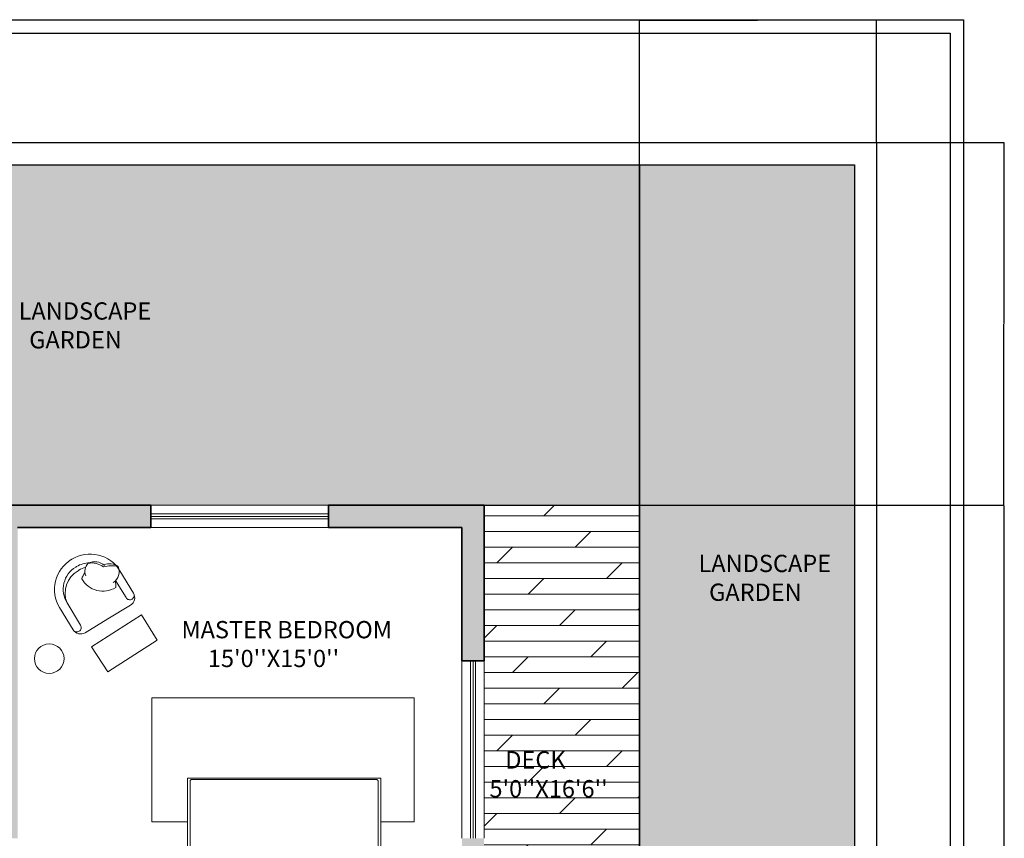
# Model space of a CAD drawing. Units: inches. Extents: x 84 to 1044, y -280 to 906.
# Tile 105 of 105: x 645 to 1044, y 574 to 906. Entities that reach past the tile are written whole.
import ezdxf

# ---------------------------------------------------------------- set-up
doc = ezdxf.new("R2010")
doc.units = ezdxf.units.IN
for name, color, linetype, lineweight in [('A-ANNO-DIMS', 2, 'Continuous', 18), ('A-ANNO-TTLB', 7, 'Continuous', 25), ('A-AREA-IDEN', 7, 'Continuous', 13), ('A-FURN', 8, 'Continuous', 15), ('C-PROP', 7, 'Continuous', 25), ('L-HRDS', 32, 'Continuous', 18), ('WALL', 250, 'Continuous', 35), ('WINDOW', 160, 'Continuous', 13)]:
    doc.layers.add(name, color=color, linetype=linetype, lineweight=lineweight)
for name, color, linetype, lineweight, true_color in [('A-FLOR-PATT', 251, 'Continuous', 9, 0x705861), ('A-WALL-PATT', 251, 'Continuous', 9, 0x636466), ('L-PLNT-PATT', 9, 'Continuous', 9, 0xafd9aa)]:
    doc.layers.add(name, color=color, linetype=linetype, lineweight=lineweight, true_color=true_color)
doc.styles.add('1-100DIM', font='txt', dxfattribs={"height": 0.3})
doc.styles.get("Standard").update_dxf_attribs({"font": 'arial.ttf'})
doc.dimstyles.get("Standard").update_dxf_attribs({"dimtxt": 0.18, "dimasz": 0.18, "dimexe": 0.18, "dimexo": 0.0625, "dimgap": 0.09, "dimtad": 0, "dimtih": 1, "dimtoh": 1, "dimdec": 4, "dimzin": 0, "dimdsep": 46, "dimtxsty": 'Standard', "dimcen": 0.09, "dimadec": 0, "dimazin": 0, "dimtfac": 1, "dimtdec": 4, "dimtofl": 0, "dimtmove": 0, "dimatfit": 3, "dimfxl": 1, "dimtolj": 1, "dimtzin": 0, "dimarcsym": 0})

# ---------------------------------------------------------------- blocks, each defined once
blk = doc.blocks.new('BED-DOUBLE-NIGHTSTANDS')
for p, q in [((33.85, 19.92), (33.85, 77.08)), ((34.63, 77.86), (109.28, 77.86)), ((110.06, 77.08), (110.06, 35.88)), ((85.85, 19.14), (110.06, 35.88)), ((88.16, 30.61), (88.22, 35.71)), ((34.63, 29.81), (88.27, 29.81)), ((88.69, 26.88), (88.16, 30.61)), ((85.85, 19.14), (34.63, 19.14)), ((47.6, 18.34), (47.89, 17.17)), ((47.89, 17.17), (48.7, 13.93)), ((75.38, 18.34), (75.67, 17.17)), ((75.67, 17.17), (76.48, 13.93)), ((32.83, 2.05), (111.17, 2.05))]:
    blk.add_line(p, q)
blk.add_lwpolyline([(111.17, 60.71), (124.69, 60.71), (124.69, 111), (18.36, 111), (18.36, 60.71), (32.83, 60.71)])
for points in [[(32.83, 78.34), (32.83, 0), (111.17, 0), (111.17, 78.34)], [(0, 23.5), (0, 0), (32.83, 0), (32.83, 23.5)], [(144, 23.5), (144, 0), (111.17, 0), (111.17, 23.5)]]:
    blk.add_lwpolyline(points, close=True)
for centre, radius, start, end in [((34.63, 77.08), 0.783, 90, 180), ((109.28, 77.08), 0.783, 0, 90), ((112.65, 181.75), 148.07, 260.505, 262.308), ((113.34, 134.29), 101.37, 258.3259, 260.505), ((119.11, 130.25), 98.54, 256.8096, 258.3259), ((98.14, 26.21), 7.6, 76.8096, 82.2696), ((100.3, 31.38), 2.28, 82.2696, 100.7276), ((136.22, -121.54), 159.21, 100.7276, 102.9255), ((113.66, 10.12), 25.75, 102.9255, 105.9352), ((129.8, -33.24), 71.88, 105.9352, 107.7364), ((34.63, 29.03), 0.783, 90, 180), ((95.31, 24.45), 7.05, 159.8512, 188.1356), ((99.64, 14.08), 14.69, 140.3555, 159.8512), ((34.63, 19.92), 0.783, 180, 270), ((47.6, 18.38), 0.0359, 265.9171, 14.0449), ((49.38, 28.85), 10.61, 260.5159, 265.9171), ((51.31, 26.86), 9, 252.6136, 260.5159), ((49.31, 13.32), 4.69, 72.6136, 83.5659), ((51.85, 12.2), 5.72, 83.5659, 101.5586), ((61.28, 45.06), 28.93, 250.572, 252.8018), ((52.93, 26.88), 9.01, 267.2509, 281.5586), ((63.4, 44.31), 28.93, 248.3423, 250.572), ((65.3, 43.56), 28.93, 246.5156, 248.3423), ((67, 42.82), 28.93, 244.6889, 246.5156), ((59.16, 72.9), 55.02, 265.3824, 267.2509), ((54.35, -29.66), 47.65, 85.3824, 87.3904), ((55.96, -113.85), 131.7, 87.3904, 89.0296), ((63.07, -206.28), 223.99, 89.0296, 90.2865), ((90.57, -34.91), 56.1, 114.3265, 116.4985), ((69.71, -27.82), 45.59, 90.2865, 93.574), ((73.97, 5.84), 12.25, 116.4985, 122.135), ((85.21, -6.34), 28.54, 122.135, 125.8263), ((70.75, 12.2), 5.71, 93.574, 102.869), ((71.21, 16.33), 1.77, 102.869, 117.2841), ((69.98, 20.94), 3.01, 286.2212, 297.2841), ((70.93, 21.67), 3.43, 277.1204, 286.2212), ((-461.55, 45.04), 534.1, 356.4951, 356.945), ((59.41, 18.76), 12.58, 350.0016, 356.4951), ((71.94, 18.4), 0.0517, 196.6978, 277.1204), ((72.69, 18.21), 0.757, 170.0016, 196.6978), ((75.38, 18.38), 0.0359, 265.9171, 14.0449), ((77.16, 28.85), 10.61, 260.5159, 265.9171), ((79.09, 26.86), 9, 252.6136, 260.5159), ((77.09, 13.32), 4.69, 72.6136, 83.5659), ((79.63, 12.2), 5.72, 83.5659, 101.5586), ((89.06, 45.06), 28.93, 250.572, 252.8018), ((80.71, 26.88), 9.01, 267.2509, 281.5586), ((91.18, 44.31), 28.93, 248.3423, 250.572), ((93.09, 43.56), 28.93, 246.5156, 248.3423), ((94.78, 42.82), 28.93, 244.6889, 246.5156), ((86.94, 72.9), 55.02, 265.3824, 267.2509), ((82.13, -29.66), 47.65, 85.3824, 87.3904), ((83.74, -113.85), 131.7, 87.3904, 89.0296), ((90.85, -206.28), 223.99, 89.0296, 90.2865), ((97.49, -27.82), 45.59, 90.2865, 93.574), ((98.54, 12.2), 5.71, 93.574, 102.869), ((98.99, 16.33), 1.77, 102.869, 117.2841), ((97.76, 20.94), 3.01, 286.2212, 297.2841), ((98.71, 21.67), 3.43, 277.1204, 286.2212), ((-433.77, 45.04), 534.1, 356.4951, 356.945), ((87.19, 18.76), 12.58, 350.0016, 356.4951), ((99.72, 18.4), 0.0517, 196.6978, 277.1204), ((100.47, 18.21), 0.757, 170.0016, 196.6978), ((74.33, 9.57), 25.8, 171.9949, 177.3351), ((51.35, 13.81), 2.65, 177.3351, 194.0452), ((63.07, 4.04), 10.66, 86.4448, 94.0828), ((64.53, 12.55), 2.27, 94.0828, 110.6743), ((72.54, -3.27), 19.85, 110.6743, 114.3265), ((18.1, 13.92), 53.48, 356.945, 358.3669), ((102.11, 9.57), 25.8, 171.9949, 177.3351), ((79.13, 13.81), 2.65, 177.3351, 194.0452), ((45.88, 13.92), 53.48, 356.945, 358.3669), ((40.12, 8.39), 7.99, 350.3156, 0), ((14.34, 15.69), 34.55, 347.8016, 350.3156), ((60.69, 8.15), 12.42, 167.8016, 171.9949), ((52.8, 8.94), 3.59, 180, 194.6851), ((51.41, 7.32), 2.2, 161.2201, 180), ((55.72, 5.76), 5.48, 152.6012, 163.485), ((56.31, 7.75), 5.48, 163.485, 174.3689), ((44.96, 9.51), 26.59, 358.3669, 3.3687), ((36.09, 3.97), 35.76, 3.3687, 7.6809), ((67.9, 8.39), 7.99, 350.3156, 0), ((42.12, 15.69), 34.55, 347.8016, 350.3156), ((88.47, 8.15), 12.42, 167.8016, 171.9949), ((72.74, 9.51), 26.59, 358.3669, 3.3687), ((63.87, 3.97), 35.76, 3.3687, 7.6809), ((46.91, 5.57), 1.34, 274.4002, 333.4195), ((46.92, 3.73), 0.514, 333.4195, 78.7276), ((28.84, 4.95), 19.27, 0, 6.2324), ((50.68, 3.26), 3.52, 126.2641, 138.5571), ((51.97, 1.08), 5.48, 117.2036, 134.9024), ((50.46, 5.22), 2.06, 138.5571, 154.6449), ((54.41, 4.38), 5.92, 154.6449, 158.1851), ((56.69, 4.33), 8.05, 158.1851, 161.2201), ((54.33, 3.44), 5.48, 134.9024, 152.6012), ((49.23, 13.22), 9.49, 277.5469, 285.744), ((51.81, 30.83), 26.74, 270, 277.5469), ((59.68, 45.18), 41.09, 263.9133, 270), ((63.35, 24.49), 20.73, 259.8101, 263.9133), ((55.99, 3.67), 7.84, 23.0028, 28.3168), ((61.71, 5.52), 1.93, 28.3168, 39.0349), ((57.3, 0.07), 8.82, 39.0349, 46.1885), ((54.63, -6.4), 15.34, 46.1885, 51.6114), ((63.87, 2), 3.01, 51.6114, 62.7604), ((62.48, -4.21), 9.17, 62.7604, 69.1397), ((62.77, 4.07), 3.89, 18.4397, 36.1766), ((64.17, 2.16), 3.89, 36.1766, 53.9136), ((66.24, 0.72), 3.89, 53.9136, 74.0648), ((64.2, 4.44), 7.77, 7.6809, 12.1095), ((81.44, 6.84), 9.64, 188.1335, 192.1095), ((73.21, 4.35), 1.28, 158.579, 188.1335), ((71.37, 3.94), 0.611, 338.579, 21.9904), ((74.69, 5.57), 1.34, 274.4002, 333.4195), ((74.7, 3.73), 0.514, 333.4195, 78.7276), ((56.62, 4.95), 19.27, 0, 6.2324), ((77.02, 13.22), 9.49, 277.5469, 285.744), ((79.59, 30.83), 26.74, 270, 277.5469), ((87.46, 45.18), 41.09, 263.9133, 270), ((91.13, 24.49), 20.73, 259.8101, 263.9133), ((83.77, 3.67), 7.84, 23.0028, 28.3168), ((89.49, 5.52), 1.93, 28.3168, 39.0349), ((85.08, 0.07), 8.82, 39.0349, 46.1885), ((82.41, -6.4), 15.34, 46.1885, 51.6114), ((91.65, 2), 3.01, 51.6114, 62.7604), ((90.26, -4.21), 9.17, 62.7604, 69.1397), ((90.56, 4.07), 3.89, 18.4397, 36.1766), ((91.95, 2.16), 3.89, 36.1766, 53.9136), ((94.02, 0.72), 3.89, 53.9136, 74.0648), ((91.98, 4.44), 7.77, 7.6809, 12.1095), ((109.22, 6.84), 9.64, 188.1335, 192.1095), ((100.99, 4.35), 1.28, 158.579, 188.1335), ((99.15, 3.94), 0.611, 338.579, 21.9904), ((47.38, -0.04), 3.54, 78.7276, 90), ((48.99, -2.82), 6.31, 90, 98.4372), ((52.23, -7.99), 11.94, 98.4372, 105.744), ((60.88, -2.08), 5.97, 79.8101, 87.4614), ((62.89, -7.52), 11.35, 87.4614, 94.8018), ((63.05, 38.02), 34.2, 270.5757, 274.8018), ((67.86, 62.44), 58.53, 268.0921, 270.5757), ((71.39, 35.92), 32.15, 264.7408, 268.0921), ((68.82, -0.02), 3.89, 74.0648, 94.2159), ((71.4, 5.61), 2.11, 239.3487, 264.7408), ((71.29, 2.38), 1.13, 59.3487, 94.3025), ((72.23, 2.44), 0.984, 94.3025, 111.7883), ((71.98, 3.55), 0.168, 21.9904, 101.8931), ((72.22, 3.59), 0.0908, 160.436, 281.8931), ((72.29, 3.37), 0.134, 111.7883, 160.436), ((75.16, -0.04), 3.54, 78.7276, 90), ((76.77, -2.82), 6.31, 90, 98.4372), ((80.01, -7.99), 11.94, 98.4372, 105.744), ((88.66, -2.08), 5.97, 79.8101, 87.4614), ((90.67, -7.52), 11.35, 87.4614, 94.8018), ((90.83, 38.02), 34.2, 270.5757, 274.8018), ((95.64, 62.44), 58.53, 268.0921, 270.5757), ((99.18, 35.92), 32.15, 264.7408, 268.0921), ((96.6, -0.02), 3.89, 74.0648, 94.2159), ((99.18, 5.61), 2.11, 239.3487, 264.7408), ((99.07, 2.38), 1.13, 59.3487, 94.3025), ((100.02, 2.44), 0.984, 94.3025, 111.7883), ((99.76, 3.55), 0.168, 21.9904, 101.8931), ((100, 3.59), 0.0908, 160.436, 281.8931), ((100.07, 3.37), 0.134, 111.7883, 160.436)]:
    blk.add_arc(centre, radius, start, end)
blk = doc.blocks.new('WIN-72IN')
for p, q in [((72, 9), (0, 9)), ((72, 5.5), (0, 5.5)), ((72, 4.5), (0, 4.5)), ((72, 3.5), (0, 3.5)), ((0, 0), (72, 0))]:
    blk.add_line(p, q)
blk = doc.blocks.new('*D62')
at = {"layer": 'A-ANNO-DIMS', "color": 0, "lineweight": -2, "transparency": 16777216}
for p, q in [((203.18, 709.18), (203.18, 905.9)), ((203.36, 905.72), (549.23, 905.72)), ((895.89, 905.72), (550.02, 905.72)), ((896.07, 400.18), (896.07, 905.9))]:
    blk.add_line(p, q, dxfattribs=at)
at = {"layer": 'A-ANNO-DIMS', "color": 0, "transparency": 16777216}
for points in [[(203.36, 905.75), (203.36, 905.69), (203.18, 905.72)], [(895.89, 905.75), (895.89, 905.69), (896.07, 905.72)]]:
    blk.add_solid(points, dxfattribs=at)
at = {"layer": 'Defpoints', "color": 0, "transparency": 16777216}
for p in [(896.07, 905.72), (203.18, 709.12), (896.07, 400.12)]:
    blk.add_point(p, dxfattribs=at)
at = {"layer": 'A-ANNO-DIMS', "color": 0, "transparency": 16777216, "insert": (549.63, 905.72), "char_height": 0.18, "attachment_point": 5}
blk.add_mtext('\\A1;692.9', dxfattribs=at)
blk = doc.blocks.new('*D63')
at = {"layer": 'A-ANNO-DIMS', "color": 0, "lineweight": -2, "transparency": 16777216}
for p, q in [((833.14, 709.12), (1043.77, 709.12)), ((1043.59, 708.94), (1043.59, 400.3)), ((1043.59, 91.3), (1043.59, 399.94)), ((896.14, 91.12), (1043.77, 91.12))]:
    blk.add_line(p, q, dxfattribs=at)
at = {"layer": 'A-ANNO-DIMS', "color": 0, "transparency": 16777216}
for points in [[(1043.56, 708.94), (1043.62, 708.94), (1043.59, 709.12)], [(1043.56, 91.3), (1043.62, 91.3), (1043.59, 91.12)]]:
    blk.add_solid(points, dxfattribs=at)
at = {"layer": 'Defpoints', "color": 0, "transparency": 16777216}
for p in [(833.07, 709.12), (1043.59, 709.12), (896.07, 91.12)]:
    blk.add_point(p, dxfattribs=at)
at = {"layer": 'A-ANNO-DIMS', "color": 0, "transparency": 16777216, "insert": (1043.59, 400.12), "char_height": 0.18, "attachment_point": 5}
blk.add_mtext('\\A1;618', dxfattribs=at)
blk = doc.blocks.new('*D65')
at = {"layer": 'A-ANNO-DIMS', "color": 0, "lineweight": -2, "transparency": 16777216}
for p, q in [((896.07, 400.18), (896.07, 905.9)), ((896.25, 905.72), (943.86, 905.72)), ((991.89, 905.72), (944.29, 905.72)), ((992.07, 856.18), (992.07, 905.9))]:
    blk.add_line(p, q, dxfattribs=at)
at = {"layer": 'A-ANNO-DIMS', "color": 0, "transparency": 16777216}
for points in [[(896.25, 905.75), (896.25, 905.69), (896.07, 905.72)], [(991.89, 905.75), (991.89, 905.69), (992.07, 905.72)]]:
    blk.add_solid(points, dxfattribs=at)
at = {"layer": 'Defpoints', "color": 0, "transparency": 16777216}
for p in [(896.07, 905.72), (992.07, 856.12), (896.07, 400.12)]:
    blk.add_point(p, dxfattribs=at)
at = {"layer": 'A-ANNO-DIMS', "color": 0, "transparency": 16777216, "insert": (944.07, 905.72), "char_height": 0.18, "attachment_point": 5}
blk.add_mtext('\\A1;96', dxfattribs=at)
blk = doc.blocks.new('*D66')
at = {"layer": 'A-ANNO-DIMS', "color": 0, "lineweight": -2, "transparency": 16777216}
for p, q in [((992.14, 856.12), (1043.77, 856.12)), ((1043.59, 855.94), (1043.59, 782.8)), ((1043.59, 709.3), (1043.59, 782.44)), ((833.14, 709.12), (1043.77, 709.12))]:
    blk.add_line(p, q, dxfattribs=at)
at = {"layer": 'A-ANNO-DIMS', "color": 0, "transparency": 16777216}
for points in [[(1043.56, 855.94), (1043.62, 855.94), (1043.59, 856.12)], [(1043.56, 709.3), (1043.62, 709.3), (1043.59, 709.12)]]:
    blk.add_solid(points, dxfattribs=at)
at = {"layer": 'Defpoints', "color": 0, "transparency": 16777216}
for p in [(992.07, 856.12), (833.07, 709.12), (1043.59, 709.12)]:
    blk.add_point(p, dxfattribs=at)
at = {"layer": 'A-ANNO-DIMS', "color": 0, "transparency": 16777216, "insert": (1043.59, 782.62), "char_height": 0.18, "attachment_point": 5}
blk.add_mtext('\\A1;147', dxfattribs=at)

msp = doc.modelspace()

# ---------------------------------------------------------------- hatches: boundary and pattern name
at = {"layer": 'A-FLOR-PATT', "transparency": 33554597}
h = msp.add_hatch(dxfattribs=at)
h.set_pattern_fill('DOLMIT', color=256)
h.paths.add_polyline_path([(896.074, 709.12), (833.074, 709.12), (833.074, 646.12), (833.074, 574.12), (833.074, 511.12), (896.074, 511.12)])
h.paths.add_polyline_path([(386.074, 769.12), (203.179, 769.12), (203.179, 709.12), (287.127, 709.12), (359.127, 709.12), (386.074, 709.12)])
at = {"layer": 'A-WALL-PATT', "transparency": 33554597}
h = msp.add_hatch(color=256, dxfattribs=at)
h.dxf.hatch_style = 1
h.paths.add_polyline_path([(671.074, 100.12), (647.074, 100.12), (647.074, 160.12), (641.074, 160.12), (620.824, 160.12), (620.824, 151.12), (638.074, 151.12), (638.074, 91.12), (671.074, 91.12)])
h.paths.add_polyline_path([(791.074, 100.12), (743.074, 100.12), (743.074, 91.12), (791.074, 91.12)])
h.paths.add_polyline_path([(896.074, 346.12), (887.074, 346.12), (887.074, 334.12), (870.955, 334.12), (833.074, 334.12), (804.574, 334.12), (804.574, 328.12), (887.074, 328.12), (887.074, 100.12), (863.074, 100.12), (863.074, 91.12), (896.074, 91.12)])
h.paths.add_polyline_path([(507.574, 154.729), (507.574, 160.12), (464.074, 160.12), (464.074, 247.12), (641.074, 247.12), (641.074, 208.12), (647.074, 208.12), (647.074, 328.12), (659.074, 328.12), (659.074, 334.12), (617.074, 334.12), (617.074, 328.12), (641.074, 328.12), (641.074, 256.12), (545.074, 256.12), (545.074, 328.12), (569.074, 328.12), (569.074, 334.12), (518.074, 334.12), (518.074, 325.12), (536.074, 325.12), (536.074, 256.12), (464.074, 256.12), (464.074, 325.12), (482.074, 325.12), (482.074, 334.12), (455.074, 334.12), (455.074, 160.12), (413.127, 160.12), (413.127, 151.12), (455.074, 151.12), (455.074, 91.12), (464.074, 91.12), (464.074, 151.12), (507.574, 151.12)])
h.paths.add_polyline_path([(572.824, 160.12), (555.574, 160.12), (555.574, 151.12), (572.824, 151.12)], flags=17)
h.paths.add_polyline_path([(341.127, 160.12), (299.179, 160.12), (299.179, 211.12), (294.179, 211.12), (290.179, 211.12), (290.179, 151.12), (341.127, 151.12)])
h.paths.add_polyline_path([(299.179, 256.12), (212.179, 256.12), (212.179, 274.12), (203.179, 274.12), (203.179, 247.12), (299.179, 247.12)])
h.paths.add_polyline_path([(212.179, 514.12), (398.074, 514.12), (398.074, 519.12), (398.074, 520.12), (212.179, 520.12), (212.179, 574.12), (203.179, 574.12), (203.179, 310.12), (212.179, 310.12), (212.179, 328.12), (290.179, 328.12), (290.179, 292.12), (299.179, 292.12), (299.179, 328.12), (332.179, 328.12), (332.179, 334.12), (212.179, 334.12)])
h.paths.add_polyline_path([(287.127, 709.12), (203.179, 709.12), (203.179, 646.12), (212.179, 646.12), (212.179, 700.12), (287.127, 700.12)])
h.paths.add_polyline_path([(470.074, 709.12), (359.127, 709.12), (359.127, 700.12), (434.074, 700.12), (434.074, 574.12), (440.074, 574.12), (440.074, 622.12), (464.074, 622.12), (464.074, 628.12), (440.074, 628.12), (440.074, 700.12), (470.074, 700.12)])
h.paths.add_polyline_path([(572.074, 709.12), (506.074, 709.12), (506.074, 700.12), (536.074, 700.12), (536.074, 628.12), (494.074, 628.12), (494.074, 622.12), (536.074, 622.12), (536.074, 520.12), (440.074, 520.12), (440.074, 544.12), (434.074, 544.12), (434.074, 514.12), (644.074, 514.12), (644.074, 519.12), (644.074, 544.12), (638.074, 544.12), (638.074, 520.12), (542.074, 520.12), (542.074, 622.12), (584.074, 622.12), (584.074, 628.12), (542.074, 628.12), (542.074, 700.12), (572.074, 700.12)])
h.paths.add_polyline_path([(698.074, 709.12), (608.074, 709.12), (608.074, 700.12), (638.074, 700.12), (638.074, 628.12), (614.074, 628.12), (614.074, 622.12), (638.074, 622.12), (638.074, 574.12), (644.074, 574.12), (644.074, 700.12), (698.074, 700.12)])
h.paths.add_polyline_path([(833.074, 709.12), (770.074, 709.12), (770.074, 700.12), (824.074, 700.12), (824.074, 646.12), (833.074, 646.12)])
h.paths.add_polyline_path([(833.074, 574.12), (824.074, 574.12), (824.074, 520.12), (791.244, 520.12), (712.904, 520.12), (680.074, 520.12), (680.074, 514.12), (695.074, 514.12), (695.074, 491.62), (704.074, 491.62), (704.074, 511.12), (833.074, 511.12)])
h.paths.add_polyline_path([(704.074, 419.62), (695.074, 419.62), (695.074, 370.12), (704.074, 370.12)])
h.paths.add_polyline_path([(896.074, 400.12), (833.074, 400.12), (833.074, 364.12), (839.074, 364.12), (839.074, 394.12), (887.074, 394.12), (887.074, 382.12), (896.074, 382.12)])
h.paths.add_polyline_path([(732.574, 334.12), (695.074, 334.12), (695.074, 328.12), (732.574, 328.12)])
at = {"layer": 'L-PLNT-PATT', "transparency": 33554597}
h = msp.add_hatch(color=256, dxfattribs=at)
h.dxf.hatch_style = 1
h.paths.add_polyline_path([(434.074, 769.12), (386.074, 769.12), (386.074, 709.12), (434.074, 709.12)])
h.paths.add_polyline_path([(896.074, 847.12), (434.074, 847.12), (434.074, 769.12), (434.074, 709.12), (470.074, 709.12), (506.074, 709.12), (572.074, 709.12), (608.074, 709.12), (698.074, 709.12), (770.074, 709.12), (833.074, 709.12), (896.074, 709.12)])
h.paths.add_polyline_path([(983.074, 847.12), (896.074, 847.12), (896.074, 709.12), (896.074, 547.12), (932.074, 547.12), (983.074, 547.12)])
h.paths.add_polyline_path([(983.074, 547.12), (932.074, 547.12), (932.074, 265.12), (983.074, 265.12)])
h.paths.add_polyline_path([(203.179, 646.12), (203.179, 709.12), (203.179, 745.12), (143.179, 745.12), (143.179, 271.12), (203.179, 271.12), (203.179, 274.12), (203.179, 310.12), (203.179, 574.12)])

# ---------------------------------------------------------------- linework, layer by layer
at = {"layer": 'A-ANNO-TTLB'}
for points in [[(101.1, 905.916), (1027.308, 905.916), (1027.308, -279.764), (101.1, -279.764)], [(106.576, 900.439), (1021.832, 900.439), (1021.832, -274.288), (106.576, -274.288)]]:
    msp.add_lwpolyline(points, close=True, dxfattribs=at)
at = {"layer": 'A-FURN'}
for points in [[(680.628, 663.048), (671.423, 657.454, -0.4142136), (666.571, 658.638), (661.068, 667.693, -0.4142136), (665.805, 687.102), (665.956, 687.193), (666.107, 687.285, -0.4142136), (685.516, 682.548), (691.018, 673.494, -0.4142136), (689.834, 668.642), (680.628, 663.048)], [(679.334, 684.712, 0.3066635), (672.647, 685.574, 0.30633), (671.703, 680.502, -0.8728472)], [(664.087, 669.527, -0.4142136), (667.639, 684.083), (667.79, 684.175)], [(664.087, 669.527, -0.3727189), (668.556, 682.574), (668.707, 682.666)], [(673.161, 685.804, 0.1305915), (667.941, 684.267), (667.79, 684.175)], [(671.628, 683.996, 0.0723842), (668.858, 682.758), (668.707, 682.666)], [(684.837, 684.222, 0.1477299), (678.85, 684.135, 0.2133428), (672.647, 685.574, 0.1786618)], [(682.824, 677.79, 0.3567724), (684.837, 684.222, 0.2495421), (679.014, 684.976, -9.6168803)], [(683.529, 678.345, -0.1655406), (683.807, 675.783, -0.4259892), (670.078, 679.278, -0.1215233), (671.366, 681.692, 7.1154643)], [(683.783, 678.599), (688, 671.66, 0.4142136), (690.426, 671.068), (690.426, 671.068, 0.4142136), (691.018, 673.494)], [(664.086, 669.527), (669.589, 660.472, -0.4142136), (668.997, 658.046), (668.997, 658.046, -0.4142136), (666.571, 658.638)]]:
    msp.add_lwpolyline(points, format="xyb", dxfattribs=at)
msp.add_lwpolyline([(674.068, 651.779), (680.633, 641.562), (700.673, 654.437), (694.26, 664.752)], close=True, dxfattribs=at)
msp.add_circle((656.87, 646.943), 6, dxfattribs=at)
at = {"layer": 'C-PROP'}
for points in [[(143.179, -121.88), (134.179, -121.88), (134.179, 856.12), (992.074, 856.12), (992.074, -121.88), (624.574, -121.88)], [(143.179, -112.88), (143.179, 847.12), (983.074, 847.12), (983.074, -112.88), (624.574, -112.88)]]:
    msp.add_lwpolyline(points, dxfattribs=at)
at = {"layer": 'L-HRDS'}
for p, q in [((896.074, 709.12), (896.074, 847.12)), ((833.074, 709.12), (896.074, 709.12)), ((896.074, 511.12), (896.074, 709.12))]:
    msp.add_line(p, q, dxfattribs=at)
at = {"layer": 'WALL'}
for p, q in [((698.074, 709.12), (608.074, 709.12)), ((698.074, 700.12), (698.074, 709.12)), ((833.074, 709.12), (770.074, 709.12)), ((770.074, 700.12), (770.074, 709.12)), ((833.074, 646.12), (833.074, 709.12)), ((698.074, 700.12), (644.074, 700.12)), ((824.074, 700.12), (770.074, 700.12)), ((824.074, 646.12), (824.074, 700.12)), ((824.074, 646.12), (833.074, 646.12))]:
    msp.add_line(p, q, dxfattribs=at)

# ---------------------------------------------------------------- block references
at = {"layer": 'A-FURN'}
msp.add_blockref('BED-DOUBLE-NIGHTSTANDS', (680.07, 520.12), dxfattribs=at)
at = {"layer": 'WINDOW'}
msp.add_blockref('WIN-72IN', (698.07, 700.12), dxfattribs=at)
at = {"layer": 'WINDOW', "rotation": 270.0000000000001}
msp.add_blockref('WIN-72IN', (824.074, 646.124), dxfattribs=at)

# ---------------------------------------------------------------- texts
at = {"layer": 'A-AREA-IDEN', "char_height": 7, "attachment_point": 1, "style": '1-100DIM'}
for s, width, insert in [('{\\f@Malgun Gothic|b0|i0|c0|p34;LANDSCAPE\\P  GARDEN}', 58.97918, (644.485, 791.351)), ('{\\f@Malgun Gothic|b0|i0|c0|p34;LANDSCAPE\\P  GARDEN}', 58.97918, (919.902, 689.031)), ("{\\f@Malgun Gothic|b0|i0|c0|p34;MASTER BEDROOM\\P     15'0''X15'0''}", 94.39973, (710.448, 662.194)), ("{\\f@Malgun Gothic|b0|i0|c0|p34;    DECK \\P 5'0''X16'6''}", 51.07953, (833.074, 609.39))]:
    msp.add_mtext_dynamic_manual_height_columns(s, width=width, gutter_width=15.851, heights=[0], dxfattribs=dict(at, insert=insert))

# ---------------------------------------------------------------- dimensions: what is measured, and where the dimension line sits
at = {"layer": 'A-ANNO-DIMS'}
for p1, override, picture, middle in [((203.179, 709.12), {"dimdec": 1, "dimlfac": 1, "dimrnd": 0, "dimzin": 0, "dimdsep": 46, "dimlunit": 2}, '*D62', (549.627, 905.72)), ((992.074, 856.12), {"dimdec": 0, "dimlfac": 1, "dimrnd": 0, "dimzin": 0, "dimdsep": 46, "dimlunit": 2}, '*D65', (944.074, 905.72))]:
    dim = msp.add_linear_dim(base=(896.074, 905.72), p1=p1, p2=(896.074, 400.12), dimstyle='Standard', override=override, dxfattribs=at)
    dim.commit()
    dim.dimension.update_dxf_attribs({"geometry": picture, "text_midpoint": middle})
for p1, picture, middle in [((992.074, 856.12), '*D66', (1043.588, 782.62)), ((896.074, 91.12), '*D63', (1043.588, 400.12))]:
    dim = msp.add_linear_dim(base=(1043.588, 709.12), p1=p1, p2=(833.074, 709.12), angle=90, dimstyle='Standard', override={"dimdec": 0, "dimlfac": 1, "dimrnd": 0, "dimzin": 0, "dimdsep": 46, "dimlunit": 2}, dxfattribs=at)
    dim.commit()
    dim.dimension.update_dxf_attribs({"geometry": picture, "text_midpoint": middle})

doc.saveas('drawing.dxf')
